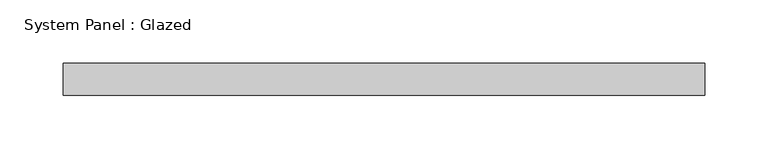
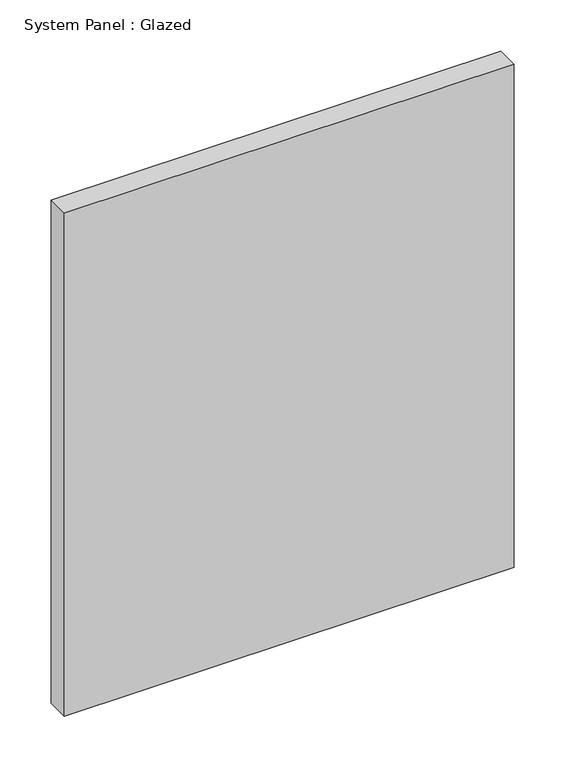
"""IFC4 building model written with IfcOpenShell, lengths in millimetres: plate geometry, System Panel : Glazed."""

from ifc_helpers import new_model, si_unit, origin, origin_with_axes, place, context, project, spatial, polyline, outline, extrude, source, transform, mapped, element, save


def system_panel_glazed_e55ceb02(model_context):
    return source(origin(), model_context, "Body", "SweptSolid", [
        extrude(outline(polyline([(254.0, 19.05), (-254.0, 19.05), (-254.0, 44.45), (254.0, 44.45), (254.0, 19.05)])), origin_with_axes(), (0.0, 0.0, 1.0), 601.3238172),
    ])


if __name__ == "__main__":
    model = new_model("IFC4")
    model_context = context("Model", 3, world=origin())
    ifc_project = project(units=[si_unit("LENGTHUNIT", "METRE", prefix="MILLI")], contexts=[model_context])
    site = spatial("IfcSite", under=ifc_project)
    building = spatial("IfcBuilding", under=site)
    placement = place(None, origin())
    system_panel_glazed_shape = system_panel_glazed_e55ceb02(model_context)
    element("IfcPlate", 1, ObjectType="System Panel : Glazed", at=placement, inside=building, context=model_context, shape_type="MappedRepresentation", body=[
        mapped(system_panel_glazed_shape, transform((0.0, 0.0, 0.0), x_axis=(1.0, 0.0, 0.0), y_axis=(0.0, 1.0, 0.0), z_axis=(0.0, 0.0, 1.0))),
    ])
    save(model, "model.ifc")

# Revit data of these elements
# Type "System Panel : Glazed"
#   Construction Type Id = "GSP4R"
#   Analytic Construction = "1/8 in Pilkington single glazing"
#   Visual Light Transmittance = 0.9
#   Solar Heat Gain Coefficient = 0.86
#   Heat Transfer Coefficient (U) = 1.18115 BTU/(h·ft²·°F)
#   Define Thermal Properties by = 1
# Element 1 (IfcPlate, "System Panel : Glazed")
#   Materials on its faces: "Glass"
# Materials
#   "Glass": class "Glass", colour RGB 0 128 192, transparency 0.75, Description = "Soda Lime Glass", Cost = 0
